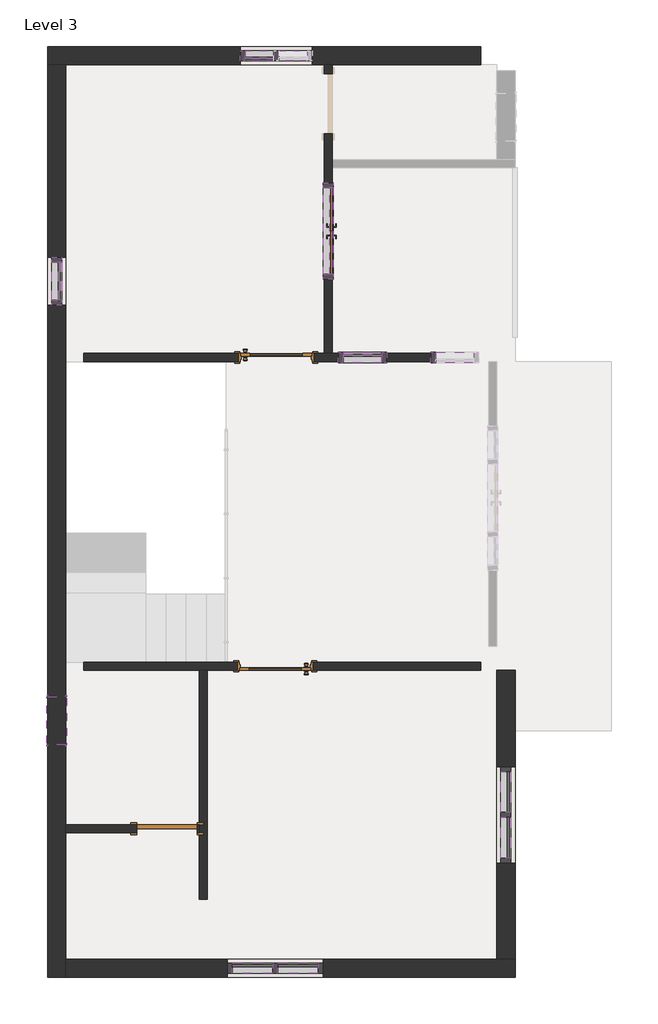
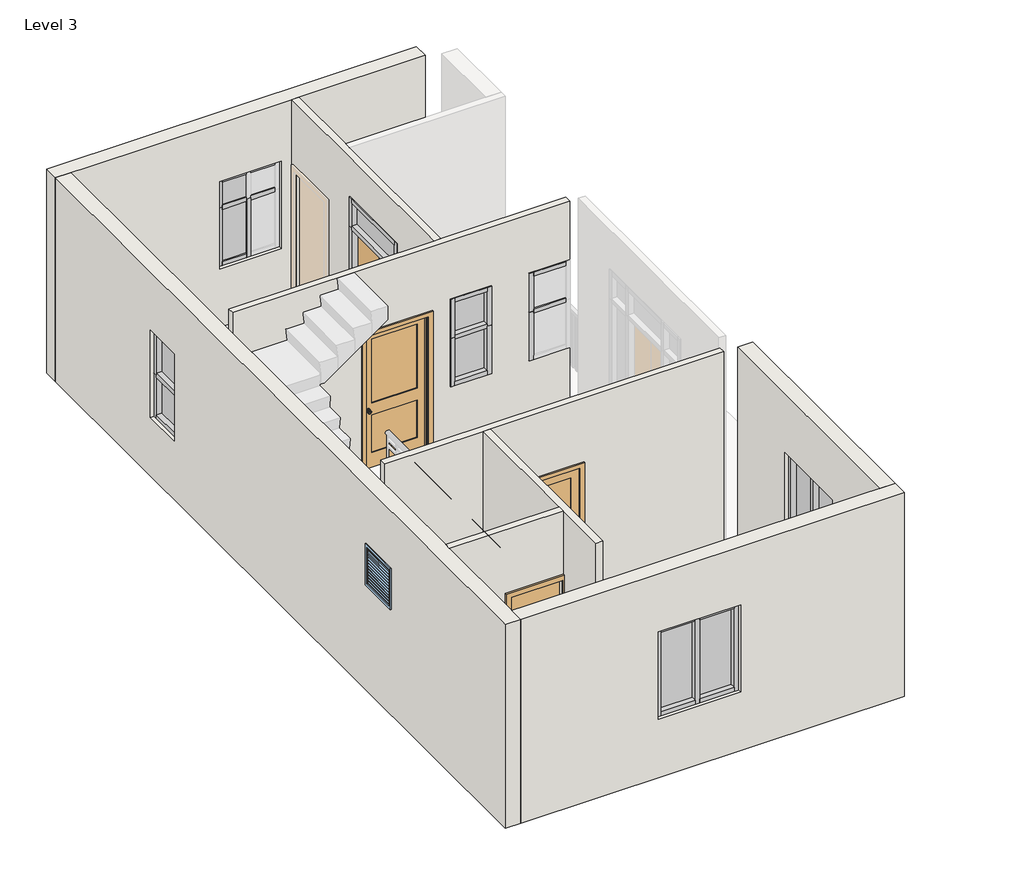
# One storey, part 1 of 2: 47 members, 11 plates, 9 walls, 4 doors, 1 window.
"""IFC4 building model written with IfcOpenShell, lengths in millimetres."""

from ifc_helpers import new_model, si_unit, frame, origin, place, context, project, spatial, polyline, outline, extrude, faceted_brep, transform, mapped, element, save
from components import door_curtain_wall_double_glass_door_curtain_wall_double_295e6296, door_interior_single_2_panel_wood_3_x7_894b38f8, door_270f2424, member_0b7646a3, member_15823cb3, member_843225dc, member_af2f84b9, member_3374d9b6, member_273a15f2, member_867fe1e1, member_86d06fe4, member_323df77c, member_47bfaf8a, member_aa870034, member_824a4a8d, member_c6627131, member_410c6227, member_73c23c35, member_6e28d7e1, system_panel_glazed_235599b7, system_panel_glazed_a38391a9, system_panel_glazed_afbb4b88, system_panel_glazed_c43f0a09, system_panel_glazed_df5e78e0, system_panel_glazed_cc98a0ec, system_panel_glazed_2bcfbbac, window_f2d8fef0

model = new_model("IFC4")

# Units and contexts
model_context = context("Model", 3, world=origin())
ifc_project = project(units=[si_unit("LENGTHUNIT", "METRE", prefix="MILLI")], contexts=[model_context])

# Site, building, storey
site = spatial("IfcSite", under=ifc_project)
building = spatial("IfcBuilding", under=site)
storey = spatial("IfcBuildingStorey", under=building, Name="Level 3", Elevation=3810.0)

# Doors
placement = place(None, origin())
door_curtain_wall_double_glass_door_curtain_wall_double_shape = door_curtain_wall_double_glass_door_curtain_wall_double_295e6296(model_context)
element("IfcDoor", 1, ObjectType="Door-Curtain-Wall-Double-Glass : Door-Curtain-Wall-Double-Glass", at=placement, inside=storey, context=model_context, shape_type="MappedRepresentation", body=[
    mapped(door_curtain_wall_double_glass_door_curtain_wall_double_shape, transform((-1506.3165653, 5261.1857557, 3873.5), x_axis=(0.0, -1.0, 0.0), y_axis=(1.0, 0.0, 0.0), z_axis=(0.0, 0.0, 1.0))),
])
door_interior_single_2_panel_wood_3_x7_shape = door_interior_single_2_panel_wood_3_x7_894b38f8(model_context)
element("IfcDoor", 2, ObjectType="Door-Interior-Single-2_Panel-Wood : 3'x7'", at=placement, inside=storey, context=model_context, shape_type="MappedRepresentation", body=[
    mapped(door_interior_single_2_panel_wood_3_x7_shape, transform((-2166.7165653, 3664.1607557, 3810.0), x_axis=(1.0, 0.0, 0.0), y_axis=(0.0, 1.0, 0.0), z_axis=(0.0, 0.0, 1.0))),
])
element("IfcDoor", 3, ObjectType="Door-Interior-Single-2_Panel-Wood : 3'x7'", at=placement, inside=storey, context=model_context, shape_type="MappedRepresentation", body=[
    mapped(door_interior_single_2_panel_wood_3_x7_shape, transform((-2179.4165653, -253.7892443, 3810.0), x_axis=(-1.0, 0.0, 0.0), y_axis=(0.0, -1.0, 0.0), z_axis=(0.0, 0.0, 1.0))),
])
door_shape = door_270f2424(model_context)
element("IfcDoor", 4, ObjectType="Single-Flush : 2'6\" x7'", at=placement, inside=storey, context=model_context, shape_type="MappedRepresentation", body=[
    mapped(door_shape, transform((-3551.0165653, -2308.0142443, 3810.0), x_axis=(1.0, 0.0, 0.0), y_axis=(0.0, 1.0, 0.0), z_axis=(0.0, 0.0, 1.0))),
])

# Members
member_shape = member_0b7646a3(model_context)
element("IfcMember", 5, ObjectType="Rectangular Mullion : 2.5\" x 5\" rectangular", at=placement, inside=storey, context=model_context, shape_type="MappedRepresentation", body=[
    mapped(member_shape, transform((741.5834347, -2676.3142441, 6096.0), x_axis=(0.0, 0.0, 1.0), y_axis=(-1.0, 0.0, 0.0), z_axis=(0.0, -1.0, 0.0))),
])
element("IfcMember", 6, ObjectType="Rectangular Mullion : 2.5\" x 5\" rectangular", at=placement, inside=storey, context=model_context, shape_type="MappedRepresentation", body=[
    mapped(member_shape, transform((741.5834347, -2098.4642441, 6096.0), x_axis=(0.0, 0.0, 1.0), y_axis=(-1.0, 0.0, 0.0), z_axis=(0.0, -1.0, 0.0))),
])
element("IfcMember", 7, ObjectType="Rectangular Mullion : 2.5\" x 5\" rectangular", at=placement, inside=storey, context=model_context, shape_type="MappedRepresentation", body=[
    mapped(member_shape, transform((-1633.3165653, -4073.3142443, 6096.0), x_axis=(0.0, 0.0, 1.0), y_axis=(0.0, -1.0, 0.0), z_axis=(1.0, 0.0, 0.0))),
])
element("IfcMember", 8, ObjectType="Rectangular Mullion : 2.5\" x 5\" rectangular", at=placement, inside=storey, context=model_context, shape_type="MappedRepresentation", body=[
    mapped(member_shape, transform((-2211.1665653, -4073.3142443, 6096.0), x_axis=(0.0, 0.0, 1.0), y_axis=(0.0, -1.0, 0.0), z_axis=(1.0, 0.0, 0.0))),
])
element("IfcMember", 9, ObjectType="Rectangular Mullion : 2.5\" x 5\" rectangular", at=placement, inside=storey, context=model_context, shape_type="MappedRepresentation", body=[
    mapped(member_shape, transform((741.5834347, -1584.1142441, 4724.4), x_axis=(0.0, 0.0, -1.0), y_axis=(-1.0, 0.0, 0.0), z_axis=(0.0, 1.0, 0.0))),
])
element("IfcMember", 10, ObjectType="Rectangular Mullion : 2.5\" x 5\" rectangular", at=placement, inside=storey, context=model_context, shape_type="MappedRepresentation", body=[
    mapped(member_shape, transform((741.5834347, -2161.9642441, 4724.4), x_axis=(0.0, 0.0, -1.0), y_axis=(-1.0, 0.0, 0.0), z_axis=(0.0, 1.0, 0.0))),
])
element("IfcMember", 11, ObjectType="Rectangular Mullion : 2.5\" x 5\" rectangular", at=placement, inside=storey, context=model_context, shape_type="MappedRepresentation", body=[
    mapped(member_shape, transform((-2725.5165653, -4073.3142443, 4724.4), x_axis=(0.0, 0.0, -1.0), y_axis=(0.0, -1.0, 0.0), z_axis=(-1.0, 0.0, 0.0))),
])
element("IfcMember", 12, ObjectType="Rectangular Mullion : 2.5\" x 5\" rectangular", at=placement, inside=storey, context=model_context, shape_type="MappedRepresentation", body=[
    mapped(member_shape, transform((-2147.6665653, -4073.3142443, 4724.4), x_axis=(0.0, 0.0, -1.0), y_axis=(0.0, -1.0, 0.0), z_axis=(-1.0, 0.0, 0.0))),
])
member_2_shape = member_15823cb3(model_context)
element("IfcMember", 13, ObjectType="Rectangular Mullion : 2.5\" x 5\" rectangular", at=placement, inside=storey, context=model_context, shape_type="MappedRepresentation", body=[
    mapped(member_2_shape, transform((-1506.3165653, 5870.7857557, 6400.8), x_axis=(0.0, 1.0, 0.0), y_axis=(-1.0, 0.0, 0.0), z_axis=(0.0, 0.0, 1.0))),
])
element("IfcMember", 14, ObjectType="Rectangular Mullion : 2.5\" x 5\" rectangular", at=placement, inside=storey, context=model_context, shape_type="MappedRepresentation", body=[
    mapped(member_2_shape, transform((-1506.3165653, 4651.5857557, 5943.6), x_axis=(0.0, -1.0, 0.0), y_axis=(-1.0, 0.0, 0.0), z_axis=(0.0, 0.0, -1.0))),
])
element("IfcMember", 15, ObjectType="Rectangular Mullion : 2.5\" x 5\" rectangular", at=placement, inside=storey, context=model_context, shape_type="MappedRepresentation", body=[
    mapped(member_2_shape, transform((-2623.9165653, 7483.6857557, 5638.8), x_axis=(-1.0, 0.0, 0.0), y_axis=(0.0, 1.0, 0.0), z_axis=(0.0, 0.0, -1.0))),
])
member_3_shape = member_843225dc(model_context)
element("IfcMember", 16, ObjectType="Rectangular Mullion : 2.5\" x 5\" rectangular", at=placement, inside=storey, context=model_context, shape_type="MappedRepresentation", body=[
    mapped(member_3_shape, transform((-2560.4165653, 7483.6857557, 6096.0), x_axis=(0.0, 0.0, 1.0), y_axis=(0.0, 1.0, 0.0), z_axis=(-1.0, 0.0, 0.0))),
])
element("IfcMember", 17, ObjectType="Rectangular Mullion : 2.5\" x 5\" rectangular", at=placement, inside=storey, context=model_context, shape_type="MappedRepresentation", body=[
    mapped(member_3_shape, transform((-2134.9665653, 7483.6857557, 6096.0), x_axis=(0.0, 0.0, 1.0), y_axis=(0.0, 1.0, 0.0), z_axis=(-1.0, 0.0, 0.0))),
])
element("IfcMember", 18, ObjectType="Rectangular Mullion : 2.5\" x 5\" rectangular", at=placement, inside=storey, context=model_context, shape_type="MappedRepresentation", body=[
    mapped(member_3_shape, transform((-2198.4665653, 7483.6857557, 4724.4), x_axis=(0.0, 0.0, -1.0), y_axis=(0.0, 1.0, 0.0), z_axis=(1.0, 0.0, 0.0))),
])
member_4_shape = member_af2f84b9(model_context)
element("IfcMember", 19, ObjectType="Rectangular Mullion : 2.5\" x 5\" rectangular", at=placement, inside=storey, context=model_context, shape_type="MappedRepresentation", body=[
    mapped(member_4_shape, transform((-2134.9665653, 7483.6857557, 5638.8), x_axis=(0.0, 0.0, 1.0), y_axis=(0.0, 1.0, 0.0), z_axis=(-1.0, 0.0, 0.0))),
])
element("IfcMember", 20, ObjectType="Rectangular Mullion : 2.5\" x 5\" rectangular", at=placement, inside=storey, context=model_context, shape_type="MappedRepresentation", body=[
    mapped(member_4_shape, transform((-2560.4165653, 7483.6857557, 5638.8), x_axis=(0.0, 0.0, 1.0), y_axis=(0.0, 1.0, 0.0), z_axis=(-1.0, 0.0, 0.0))),
])
member_5_shape = member_3374d9b6(model_context)
element("IfcMember", 21, ObjectType="Rectangular Mullion : 2.5\" x 5\" rectangular", at=placement, inside=storey, context=model_context, shape_type="MappedRepresentation", body=[
    mapped(member_5_shape, transform((-1506.3165653, 4651.5857557, 3810.0), x_axis=(0.0, -1.0, 0.0), y_axis=(-1.0, 0.0, 0.0), z_axis=(0.0, 0.0, -1.0))),
])
element("IfcMember", 22, ObjectType="Rectangular Mullion : 2.5\" x 5\" rectangular", at=placement, inside=storey, context=model_context, shape_type="MappedRepresentation", body=[
    mapped(member_5_shape, transform((-1506.3165653, 5870.7857557, 5943.6), x_axis=(0.0, 1.0, 0.0), y_axis=(-1.0, 0.0, 0.0), z_axis=(0.0, 0.0, 1.0))),
])
member_6_shape = member_273a15f2(model_context)
element("IfcMember", 23, ObjectType="Rectangular Mullion : 2.5\" x 5\" rectangular", at=placement, inside=storey, context=model_context, shape_type="MappedRepresentation", body=[
    mapped(member_6_shape, transform((-1506.3165653, 4715.0857557, 6400.8), x_axis=(0.0, 0.0, 1.0), y_axis=(-1.0, 0.0, 0.0), z_axis=(0.0, -1.0, 0.0))),
])
element("IfcMember", 24, ObjectType="Rectangular Mullion : 2.5\" x 5\" rectangular", at=placement, inside=storey, context=model_context, shape_type="MappedRepresentation", body=[
    mapped(member_6_shape, transform((-1506.3165653, 5807.2857557, 3810.0), x_axis=(0.0, 0.0, -1.0), y_axis=(-1.0, 0.0, 0.0), z_axis=(0.0, 1.0, 0.0))),
])
member_7_shape = member_867fe1e1(model_context)
element("IfcMember", 25, ObjectType="Rectangular Mullion : 2.5\" x 5\" rectangular", at=placement, inside=storey, context=model_context, shape_type="MappedRepresentation", body=[
    mapped(member_7_shape, transform((-1506.3165653, 4715.0857557, 5943.6), x_axis=(0.0, 0.0, 1.0), y_axis=(-1.0, 0.0, 0.0), z_axis=(0.0, -1.0, 0.0))),
])
member_8_shape = member_86d06fe4(model_context)
element("IfcMember", 26, ObjectType="Rectangular Mullion : 2.5\" x 5\" rectangular", at=placement, inside=storey, context=model_context, shape_type="MappedRepresentation", body=[
    mapped(member_8_shape, transform((-147.4165653, 3660.9857557, 6096.0), x_axis=(0.0, 0.0, 1.0), y_axis=(0.0, 1.0, 0.0), z_axis=(-1.0, 0.0, 0.0))),
])
element("IfcMember", 27, ObjectType="Rectangular Mullion : 2.5\" x 5\" rectangular", at=placement, inside=storey, context=model_context, shape_type="MappedRepresentation", body=[
    mapped(member_8_shape, transform((-833.2165653, 3660.9857557, 6096.0), x_axis=(0.0, 0.0, 1.0), y_axis=(0.0, -1.0, 0.0), z_axis=(1.0, 0.0, 0.0))),
])
element("IfcMember", 28, ObjectType="Rectangular Mullion : 2.5\" x 5\" rectangular", at=placement, inside=storey, context=model_context, shape_type="MappedRepresentation", body=[
    mapped(member_8_shape, transform((-4948.0165653, 4384.8857559, 6096.0), x_axis=(0.0, 0.0, 1.0), y_axis=(-1.0, 0.0, 0.0), z_axis=(0.0, -1.0, 0.0))),
])
element("IfcMember", 29, ObjectType="Rectangular Mullion : 2.5\" x 5\" rectangular", at=placement, inside=storey, context=model_context, shape_type="MappedRepresentation", body=[
    mapped(member_8_shape, transform((-1315.8165653, 3660.9857557, 4724.4), x_axis=(0.0, 0.0, -1.0), y_axis=(0.0, -1.0, 0.0), z_axis=(-1.0, 0.0, 0.0))),
])
element("IfcMember", 30, ObjectType="Rectangular Mullion : 2.5\" x 5\" rectangular", at=placement, inside=storey, context=model_context, shape_type="MappedRepresentation", body=[
    mapped(member_8_shape, transform((-4948.0165653, 4867.4857559, 4724.4), x_axis=(0.0, 0.0, -1.0), y_axis=(-1.0, 0.0, 0.0), z_axis=(0.0, 1.0, 0.0))),
])
member_9_shape = member_323df77c(model_context)
element("IfcMember", 31, ObjectType="Rectangular Mullion : 2.5\" x 5\" rectangular", at=placement, inside=storey, context=model_context, shape_type="MappedRepresentation", body=[
    mapped(member_9_shape, transform((-147.4165653, 3660.9857557, 5486.4), x_axis=(0.0, 0.0, 1.0), y_axis=(0.0, 1.0, 0.0), z_axis=(-1.0, 0.0, 0.0))),
])
element("IfcMember", 32, ObjectType="Rectangular Mullion : 2.5\" x 5\" rectangular", at=placement, inside=storey, context=model_context, shape_type="MappedRepresentation", body=[
    mapped(member_9_shape, transform((-833.2165653, 3660.9857557, 5486.4), x_axis=(0.0, 0.0, 1.0), y_axis=(0.0, -1.0, 0.0), z_axis=(1.0, 0.0, 0.0))),
])
element("IfcMember", 33, ObjectType="Rectangular Mullion : 2.5\" x 5\" rectangular", at=placement, inside=storey, context=model_context, shape_type="MappedRepresentation", body=[
    mapped(member_9_shape, transform((-4948.0165653, 4384.8857559, 5410.2), x_axis=(0.0, 0.0, 1.0), y_axis=(-1.0, 0.0, 0.0), z_axis=(0.0, -1.0, 0.0))),
])
member_10_shape = member_47bfaf8a(model_context)
element("IfcMember", 34, ObjectType="Rectangular Mullion : 2.5\" x 5\" rectangular", at=placement, inside=storey, context=model_context, shape_type="MappedRepresentation", body=[
    mapped(member_10_shape, transform((-1379.3165653, 3660.9857557, 6096.0), x_axis=(-1.0, 0.0, 0.0), y_axis=(0.0, -1.0, 0.0), z_axis=(0.0, 0.0, 1.0))),
])
member_11_shape = member_aa870034(model_context)
element("IfcMember", 35, ObjectType="Rectangular Mullion : 2.5\" x 5\" rectangular", at=placement, inside=storey, context=model_context, shape_type="MappedRepresentation", body=[
    mapped(member_11_shape, transform((-210.9165653, 3660.9857557, 4724.4), x_axis=(-1.0, 0.0, 0.0), y_axis=(0.0, 1.0, 0.0), z_axis=(0.0, 0.0, -1.0))),
])
element("IfcMember", 36, ObjectType="Rectangular Mullion : 2.5\" x 5\" rectangular", at=placement, inside=storey, context=model_context, shape_type="MappedRepresentation", body=[
    mapped(member_11_shape, transform((-769.7165653, 3660.9857557, 4724.4), x_axis=(1.0, 0.0, 0.0), y_axis=(0.0, -1.0, 0.0), z_axis=(0.0, 0.0, -1.0))),
])
element("IfcMember", 37, ObjectType="Rectangular Mullion : 2.5\" x 5\" rectangular", at=placement, inside=storey, context=model_context, shape_type="MappedRepresentation", body=[
    mapped(member_10_shape, transform((-210.9165653, 3660.9857557, 5486.4), x_axis=(-1.0, 0.0, 0.0), y_axis=(0.0, 1.0, 0.0), z_axis=(0.0, 0.0, -1.0))),
])
element("IfcMember", 38, ObjectType="Rectangular Mullion : 2.5\" x 5\" rectangular", at=placement, inside=storey, context=model_context, shape_type="MappedRepresentation", body=[
    mapped(member_10_shape, transform((-769.7165653, 3660.9857557, 5486.4), x_axis=(1.0, 0.0, 0.0), y_axis=(0.0, -1.0, 0.0), z_axis=(0.0, 0.0, -1.0))),
])
element("IfcMember", 39, ObjectType="Rectangular Mullion : 2.5\" x 5\" rectangular", at=placement, inside=storey, context=model_context, shape_type="MappedRepresentation", body=[
    mapped(member_11_shape, transform((-1379.3165653, 3660.9857557, 5486.4), x_axis=(-1.0, 0.0, 0.0), y_axis=(0.0, -1.0, 0.0), z_axis=(0.0, 0.0, 1.0))),
])
member_12_shape = member_824a4a8d(model_context)
element("IfcMember", 40, ObjectType="Rectangular Mullion : 2.5\" x 5\" rectangular", at=placement, inside=storey, context=model_context, shape_type="MappedRepresentation", body=[
    mapped(member_12_shape, transform((741.5834347, -2130.2142441, 4724.4), x_axis=(0.0, -1.0, 0.0), y_axis=(-1.0, 0.0, 0.0), z_axis=(0.0, 0.0, -1.0))),
])
element("IfcMember", 41, ObjectType="Rectangular Mullion : 2.5\" x 5\" rectangular", at=placement, inside=storey, context=model_context, shape_type="MappedRepresentation", body=[
    mapped(member_12_shape, transform((-2179.4165653, -4073.3142443, 4724.4), x_axis=(1.0, 0.0, 0.0), y_axis=(0.0, -1.0, 0.0), z_axis=(0.0, 0.0, -1.0))),
])
member_13_shape = member_c6627131(model_context)
element("IfcMember", 42, ObjectType="Rectangular Mullion : 2.5\" x 5\" rectangular", at=placement, inside=storey, context=model_context, shape_type="MappedRepresentation", body=[
    mapped(member_13_shape, transform((741.5834347, -1520.6142441, 6096.0), x_axis=(0.0, 1.0, 0.0), y_axis=(-1.0, 0.0, 0.0), z_axis=(0.0, 0.0, 1.0))),
])
element("IfcMember", 43, ObjectType="Rectangular Mullion : 2.5\" x 5\" rectangular", at=placement, inside=storey, context=model_context, shape_type="MappedRepresentation", body=[
    mapped(member_13_shape, transform((-2789.0165653, -4073.3142443, 6096.0), x_axis=(-1.0, 0.0, 0.0), y_axis=(0.0, -1.0, 0.0), z_axis=(0.0, 0.0, 1.0))),
])
element("IfcMember", 44, ObjectType="Rectangular Mullion : 2.5\" x 5\" rectangular", at=placement, inside=storey, context=model_context, shape_type="MappedRepresentation", body=[
    mapped(member_13_shape, transform((741.5834347, -2739.8142441, 4724.4), x_axis=(0.0, -1.0, 0.0), y_axis=(-1.0, 0.0, 0.0), z_axis=(0.0, 0.0, -1.0))),
])
element("IfcMember", 45, ObjectType="Rectangular Mullion : 2.5\" x 5\" rectangular", at=placement, inside=storey, context=model_context, shape_type="MappedRepresentation", body=[
    mapped(member_13_shape, transform((-1569.8165653, -4073.3142443, 4724.4), x_axis=(1.0, 0.0, 0.0), y_axis=(0.0, -1.0, 0.0), z_axis=(0.0, 0.0, -1.0))),
])
member_14_shape = member_410c6227(model_context)
element("IfcMember", 46, ObjectType="Rectangular Mullion : 2.5\" x 5\" rectangular", at=placement, inside=storey, context=model_context, shape_type="MappedRepresentation", body=[
    mapped(member_14_shape, transform((-2166.7165653, 7483.6857557, 4724.4), x_axis=(-1.0, 0.0, 0.0), y_axis=(0.0, 1.0, 0.0), z_axis=(0.0, 0.0, -1.0))),
])
member_15_shape = member_73c23c35(model_context)
element("IfcMember", 47, ObjectType="Rectangular Mullion : 2.5\" x 5\" rectangular", at=placement, inside=storey, context=model_context, shape_type="MappedRepresentation", body=[
    mapped(member_15_shape, transform((-2623.9165653, 7483.6857557, 4724.4), x_axis=(-1.0, 0.0, 0.0), y_axis=(0.0, 1.0, 0.0), z_axis=(0.0, 0.0, -1.0))),
])
member_16_shape = member_6e28d7e1(model_context)
element("IfcMember", 48, ObjectType="Rectangular Mullion : 2.5\" x 5\" rectangular", at=placement, inside=storey, context=model_context, shape_type="MappedRepresentation", body=[
    mapped(member_16_shape, transform((-4948.0165653, 4930.9857559, 6096.0), x_axis=(0.0, 1.0, 0.0), y_axis=(-1.0, 0.0, 0.0), z_axis=(0.0, 0.0, 1.0))),
])
element("IfcMember", 49, ObjectType="Rectangular Mullion : 2.5\" x 5\" rectangular", at=placement, inside=storey, context=model_context, shape_type="MappedRepresentation", body=[
    mapped(member_16_shape, transform((-4948.0165653, 4321.3857559, 4724.4), x_axis=(0.0, -1.0, 0.0), y_axis=(-1.0, 0.0, 0.0), z_axis=(0.0, 0.0, -1.0))),
])
element("IfcMember", 50, ObjectType="Rectangular Mullion : 2.5\" x 5\" rectangular", at=placement, inside=storey, context=model_context, shape_type="MappedRepresentation", body=[
    mapped(member_16_shape, transform((-4948.0165653, 4321.3857559, 5410.2), x_axis=(0.0, -1.0, 0.0), y_axis=(-1.0, 0.0, 0.0), z_axis=(0.0, 0.0, -1.0))),
])
element("IfcMember", 51, ObjectType="Rectangular Mullion : 2.5\" x 5\" rectangular", at=placement, inside=storey, context=model_context, shape_type="MappedRepresentation", body=[
    mapped(member_16_shape, transform((-4948.0165653, 4930.9857559, 5410.2), x_axis=(0.0, 1.0, 0.0), y_axis=(-1.0, 0.0, 0.0), z_axis=(0.0, 0.0, 1.0))),
])

# Plates
system_panel_glazed_shape = system_panel_glazed_235599b7(model_context)
element("IfcPlate", 52, ObjectType="System Panel : Glazed", at=placement, inside=storey, context=model_context, shape_type="MappedRepresentation", body=[
    mapped(system_panel_glazed_shape, transform((-2379.4415653, 7483.6857557, 5670.55), x_axis=(-1.0, 0.0, 0.0), y_axis=(0.0, -1.0, 0.0), z_axis=(0.0, 0.0, 1.0))),
])
system_panel_glazed_2_shape = system_panel_glazed_a38391a9(model_context)
element("IfcPlate", 53, ObjectType="System Panel : Glazed", at=placement, inside=storey, context=model_context, shape_type="MappedRepresentation", body=[
    mapped(system_panel_glazed_2_shape, transform((-1506.3165653, 5261.1857557, 5975.35), x_axis=(0.0, -1.0, 0.0), y_axis=(1.0, 0.0, 0.0), z_axis=(0.0, 0.0, 1.0))),
])
system_panel_glazed_3_shape = system_panel_glazed_afbb4b88(model_context)
element("IfcPlate", 54, ObjectType="System Panel : Glazed", at=placement, inside=storey, context=model_context, shape_type="MappedRepresentation", body=[
    mapped(system_panel_glazed_3_shape, transform((-1074.5165653, 3660.9857557, 4787.9), x_axis=(1.0, 0.0, 0.0), y_axis=(0.0, 1.0, 0.0), z_axis=(0.0, 0.0, 1.0))),
])
system_panel_glazed_4_shape = system_panel_glazed_c43f0a09(model_context)
element("IfcPlate", 55, ObjectType="System Panel : Glazed", at=placement, inside=storey, context=model_context, shape_type="MappedRepresentation", body=[
    mapped(system_panel_glazed_4_shape, transform((-1074.5165653, 3660.9857557, 5518.15), x_axis=(1.0, 0.0, 0.0), y_axis=(0.0, 1.0, 0.0), z_axis=(0.0, 0.0, 1.0))),
])
system_panel_glazed_5_shape = system_panel_glazed_df5e78e0(model_context)
element("IfcPlate", 56, ObjectType="System Panel : Glazed", at=placement, inside=storey, context=model_context, shape_type="MappedRepresentation", body=[
    mapped(system_panel_glazed_5_shape, transform((741.5834347, -1841.2892441, 4787.9), x_axis=(0.0, -1.0, 0.0), y_axis=(1.0, 0.0, 0.0), z_axis=(0.0, 0.0, 1.0))),
])
element("IfcPlate", 57, ObjectType="System Panel : Glazed", at=placement, inside=storey, context=model_context, shape_type="MappedRepresentation", body=[
    mapped(system_panel_glazed_5_shape, transform((-2468.3415653, -4073.3142443, 4787.9), x_axis=(1.0, 0.0, 0.0), y_axis=(0.0, 1.0, 0.0), z_axis=(0.0, 0.0, 1.0))),
])
element("IfcPlate", 58, ObjectType="System Panel : Glazed", at=placement, inside=storey, context=model_context, shape_type="MappedRepresentation", body=[
    mapped(system_panel_glazed_5_shape, transform((-1890.4915653, -4073.3142443, 4787.9), x_axis=(1.0, 0.0, 0.0), y_axis=(0.0, 1.0, 0.0), z_axis=(0.0, 0.0, 1.0))),
])
element("IfcPlate", 59, ObjectType="System Panel : Glazed", at=placement, inside=storey, context=model_context, shape_type="MappedRepresentation", body=[
    mapped(system_panel_glazed_5_shape, transform((741.5834347, -2419.1392441, 4787.9), x_axis=(0.0, -1.0, 0.0), y_axis=(1.0, 0.0, 0.0), z_axis=(0.0, 0.0, 1.0))),
])
system_panel_glazed_6_shape = system_panel_glazed_cc98a0ec(model_context)
element("IfcPlate", 60, ObjectType="System Panel : Glazed", at=placement, inside=storey, context=model_context, shape_type="MappedRepresentation", body=[
    mapped(system_panel_glazed_6_shape, transform((-2379.4415653, 7483.6857557, 4787.9), x_axis=(-1.0, 0.0, 0.0), y_axis=(0.0, -1.0, 0.0), z_axis=(0.0, 0.0, 1.0))),
])
system_panel_glazed_7_shape = system_panel_glazed_2bcfbbac(model_context)
element("IfcPlate", 61, ObjectType="System Panel : Glazed", at=placement, inside=storey, context=model_context, shape_type="MappedRepresentation", body=[
    mapped(system_panel_glazed_7_shape, transform((-4948.0165653, 4626.1857559, 4787.9), x_axis=(0.0, -1.0, 0.0), y_axis=(1.0, 0.0, 0.0), z_axis=(0.0, 0.0, 1.0))),
])
element("IfcPlate", 62, ObjectType="System Panel : Glazed", at=placement, inside=storey, context=model_context, shape_type="MappedRepresentation", body=[
    mapped(system_panel_glazed_7_shape, transform((-4948.0165653, 4626.1857559, 5441.95), x_axis=(0.0, -1.0, 0.0), y_axis=(1.0, 0.0, 0.0), z_axis=(0.0, 0.0, 1.0))),
])

# Walls
element("IfcWall", 63, at=placement, inside=storey, context=model_context, shape_type="Brep", body=[
    faceted_brep([(398.6834347, 3610.1857557, 7010.4), (-4605.1165653, 3610.1857557, 7010.4), (-4605.1165653, 3610.1857557, 3810.0), (-2649.3165653, 3610.1857557, 3810.0), (-2649.3165653, 3610.1857557, 5969.0), (-1684.1165653, 3610.1857557, 5969.0), (-1684.1165653, 3610.1857557, 3810.0), (398.6834347, 3610.1857557, 3810.0), (398.6834347, 3610.1857557, 4724.4), (-210.9165653, 3610.1857557, 4724.4), (-210.9165653, 3610.1857557, 6096.0), (398.6834347, 3610.1857557, 6096.0), (-1379.3165653, 3610.1857557, 4724.4), (-1379.3165653, 3610.1857557, 6096.0), (-769.7165653, 3610.1857557, 6096.0), (-769.7165653, 3610.1857557, 4724.4), (-4605.1165653, 3711.7857557, 7010.4), (-1557.1165653, 3711.7857557, 7010.4), (-1455.5165653, 3711.7857557, 7010.4), (398.6834347, 3711.7857557, 7010.4), (398.6834347, 3711.7857557, 6096.0), (-210.9165653, 3711.7857557, 6096.0), (-210.9165653, 3711.7857557, 4724.4), (398.6834347, 3711.7857557, 4724.4), (398.6834347, 3711.7857557, 3810.0), (-1455.5165653, 3711.7857557, 3810.0), (-1557.1165653, 3711.7857557, 3810.0), (-1684.1165653, 3711.7857557, 3810.0), (-1684.1165653, 3711.7857557, 5969.0), (-2649.3165653, 3711.7857557, 5969.0), (-2649.3165653, 3711.7857557, 3810.0), (-4605.1165653, 3711.7857557, 3810.0), (-1379.3165653, 3711.7857557, 6096.0), (-1379.3165653, 3711.7857557, 4724.4), (-769.7165653, 3711.7857557, 4724.4), (-769.7165653, 3711.7857557, 6096.0)], [[[0, 1, 2, 3, 4, 5, 6, 7, 8, 9, 10, 11], [12, 13, 14, 15]], [[16, 17, 18, 19, 20, 21, 22, 23, 24, 25, 26, 27, 28, 29, 30, 31], [32, 33, 34, 35]], [[2, 31, 30, 3]], [[24, 7, 6, 27, 26, 25]], [[7, 24, 23, 8]], [[19, 0, 11, 20]], [[1, 0, 19, 18, 17, 16]], [[2, 1, 16, 31]], [[5, 28, 27, 6]], [[28, 5, 4, 29]], [[29, 4, 3, 30]], [[12, 33, 32, 13]], [[13, 32, 35, 14]], [[34, 15, 14, 35]], [[33, 12, 15, 34]], [[10, 21, 20, 11]], [[21, 10, 9, 22]], [[22, 9, 8, 23]]]),
])
element("IfcWall", 64, at=placement, inside=storey, context=model_context, shape_type="Brep", body=[
    faceted_brep([(424.0834347, -301.4142443, 3810.0), (424.0834347, -301.4142443, 7010.4), (-3043.0165653, -301.4142443, 7010.4), (-3144.6165653, -301.4142443, 7010.4), (-4605.1165653, -301.4142443, 7010.4), (-4605.1165653, -301.4142443, 3810.0), (-3144.6165653, -301.4142443, 3810.0), (-3043.0165653, -301.4142443, 3810.0), (-2662.0165653, -301.4142443, 3810.0), (-2662.0165653, -301.4142443, 5969.0), (-1696.8165653, -301.4142443, 5969.0), (-1696.8165653, -301.4142443, 3810.0), (398.6834347, -301.4142443, 3810.0), (424.0834347, -199.8142443, 7010.4), (424.0834347, -199.8142443, 3810.0), (398.6834347, -199.8142443, 3810.0), (-1696.8165653, -199.8142443, 3810.0), (-1696.8165653, -199.8142443, 5969.0), (-2662.0165653, -199.8142443, 5969.0), (-2662.0165653, -199.8142443, 3810.0), (-4605.1165653, -199.8142443, 3810.0), (-4605.1165653, -199.8142443, 7010.4), (398.6834347, -199.8142443, 7010.4)], [[[0, 1, 2, 3, 4, 5, 6, 7, 8, 9, 10, 11, 12]], [[13, 14, 15, 16, 17, 18, 19, 20, 21, 22]], [[5, 20, 19, 8, 7, 6]], [[14, 0, 12, 11, 16, 15]], [[1, 0, 14, 13]], [[4, 3, 2, 1, 13, 22, 21]], [[5, 4, 21, 20]], [[18, 9, 8, 19]], [[9, 18, 17, 10]], [[10, 17, 16, 11]]]),
])
element("IfcWall", 65, at=placement, inside=storey, context=model_context, shape_type="Brep", body=[
    faceted_brep([(-1455.5165653, 7369.3857557, 7010.4), (-1455.5165653, 6162.8857557, 7010.4), (-1455.5165653, 6061.2857557, 7010.4), (-1455.5165653, 3711.7857557, 7010.4), (-1455.5165653, 3711.7857557, 3810.0), (-1455.5165653, 4651.5857557, 3810.0), (-1455.5165653, 4651.5857557, 6400.8), (-1455.5165653, 5870.7857557, 6400.8), (-1455.5165653, 5870.7857557, 3810.0), (-1455.5165653, 6061.2857557, 3810.0), (-1455.5165653, 6162.8857557, 3810.0), (-1455.5165653, 6493.0857557, 3810.0), (-1455.5165653, 6493.0857557, 5943.6), (-1455.5165653, 7255.0857557, 5943.6), (-1455.5165653, 7255.0857557, 3810.0), (-1455.5165653, 7369.3857557, 3810.0), (-1557.1165653, 3711.7857557, 7010.4), (-1557.1165653, 7369.3857557, 7010.4), (-1557.1165653, 7369.3857557, 3810.0), (-1557.1165653, 7255.0857557, 3810.0), (-1557.1165653, 7255.0857557, 5943.6), (-1557.1165653, 6493.0857557, 5943.6), (-1557.1165653, 6493.0857557, 3810.0), (-1557.1165653, 5870.7857557, 3810.0), (-1557.1165653, 5870.7857557, 6400.8), (-1557.1165653, 4651.5857557, 6400.8), (-1557.1165653, 4651.5857557, 3810.0), (-1557.1165653, 3711.7857557, 3810.0)], [[[0, 1, 2, 3, 4, 5, 6, 7, 8, 9, 10, 11, 12, 13, 14, 15]], [[16, 17, 18, 19, 20, 21, 22, 23, 24, 25, 26, 27]], [[4, 27, 26, 5]], [[18, 15, 14, 19]], [[22, 11, 10, 9, 8, 23]], [[3, 2, 1, 0, 17, 16]], [[4, 3, 16, 27]], [[0, 15, 18, 17]], [[20, 19, 14, 13]], [[21, 20, 13, 12]], [[22, 21, 12, 11]], [[7, 24, 23, 8]], [[24, 7, 6, 25]], [[25, 6, 5, 26]]]),
])
element("IfcWall", 66, at=placement, inside=storey, context=model_context, shape_type="Brep", body=[
    faceted_brep([(-3144.6165653, -301.4142443, 3810.0), (-3144.6165653, -2257.2142443, 3810.0), (-3144.6165653, -2358.8142443, 3810.0), (-3144.6165653, -3197.0142443, 3810.0), (-3144.6165653, -3197.0142443, 7010.4), (-3144.6165653, -2358.8142443, 7010.4), (-3144.6165653, -2257.2142443, 7010.4), (-3144.6165653, -301.4142443, 7010.4), (-3043.0165653, -301.4142443, 3810.0), (-3043.0165653, -301.4142443, 7010.4), (-3043.0165653, -3197.0142443, 7010.4), (-3043.0165653, -3197.0142443, 3810.0)], [[[0, 1, 2, 3, 4, 5, 6, 7]], [[8, 9, 10, 11]], [[3, 2, 1, 0, 8, 11]], [[4, 3, 11, 10]], [[7, 6, 5, 4, 10, 9]], [[0, 7, 9, 8]]]),
])
element("IfcWall", 67, at=placement, inside=storey, context=model_context, shape_type="SweptSolid", body=[
    extrude(outline(polyline([(5943.6, -3170.0165653), (3810.0, -3170.0165653), (3810.0, -3144.6165653), (7010.4, -3144.6165653), (7010.4, -4833.7165653), (3810.0, -4833.7165653), (3810.0, -3932.0165653), (5943.6, -3932.0165653), (5943.6, -3170.0165653)])), frame((0.0, -2358.8142443, 0.0), z_axis=(0.0, 1.0, 0.0), x_axis=(0.0, 0.0, 1.0)), (0.0, 0.0, 1.0), 101.6),
])
element("IfcWall", 68, ObjectType="9\" wall", at=placement, inside=storey, context=model_context, shape_type="Brep", body=[
    faceted_brep([(-5062.3165653, 7369.3857557, 3810.0), (-4833.7165653, 7369.3857557, 3810.0), (-1557.1165653, 7369.3857557, 3810.0), (-1455.5165653, 7369.3857557, 3810.0), (398.6834347, 7369.3857557, 3810.0), (424.0834347, 7369.3857557, 3810.0), (424.0834347, 7369.3857557, 7010.4), (398.6834347, 7369.3857557, 7010.4), (-1455.5165653, 7369.3857557, 7010.4), (-1557.1165653, 7369.3857557, 7010.4), (-4605.1165653, 7369.3857557, 7010.4), (-4833.7165653, 7369.3857557, 7010.4), (-5062.3165653, 7369.3857557, 7010.4), (-1709.5165653, 7369.3857557, 6096.0), (-1709.5165653, 7369.3857557, 4724.4), (-2623.9165653, 7369.3857557, 4724.4), (-2623.9165653, 7369.3857557, 6096.0), (424.0834347, 7597.9857557, 3810.0), (398.6834347, 7597.9857557, 3810.0), (-5062.3165653, 7597.9857557, 3810.0), (-5062.3165653, 7597.9857557, 7010.4), (424.0834347, 7597.9857557, 7010.4), (-1709.5165653, 7597.9857557, 4724.4), (-1709.5165653, 7597.9857557, 6096.0), (-2623.9165653, 7597.9857557, 6096.0), (-2623.9165653, 7597.9857557, 4724.4)], [[[0, 1, 2, 3, 4, 5, 6, 7, 8, 9, 10, 11, 12], [13, 14, 15, 16]], [[17, 18, 19, 20, 21], [22, 23, 24, 25]], [[5, 4, 3, 2, 1, 0, 19, 18, 17]], [[6, 5, 17, 21]], [[12, 11, 10, 9, 8, 7, 6, 21, 20]], [[0, 12, 20, 19]], [[22, 14, 13, 23]], [[23, 13, 16, 24]], [[24, 16, 15, 25]], [[14, 22, 25, 15]]]),
])
element("IfcWall", 69, ObjectType="9\" wall", at=placement, inside=storey, context=model_context, shape_type="Brep", body=[
    faceted_brep([(-5062.3165653, 7369.3857557, 3810.0), (-5062.3165653, -4187.6142443, 3810.0), (-5062.3165653, -4187.6142443, 7010.4), (-5062.3165653, 7369.3857557, 7010.4), (-5062.3165653, 4930.9857559, 4724.4), (-5062.3165653, 4930.9857559, 6096.0), (-5062.3165653, 4321.3857559, 6096.0), (-5062.3165653, 4321.3857559, 4724.4), (-5062.3165653, -1241.2142443, 6096.0), (-5062.3165653, -1241.2142443, 5486.4), (-5062.3165653, -631.6142443, 5486.4), (-5062.3165653, -631.6142443, 6096.0), (-4833.7165653, -4187.6142443, 3810.0), (-4833.7165653, -3959.0142443, 3810.0), (-4833.7165653, -2358.8142443, 3810.0), (-4833.7165653, -2257.2142443, 3810.0), (-4833.7165653, -301.4142443, 3810.0), (-4833.7165653, -199.8142443, 3810.0), (-4833.7165653, 3610.1857557, 3810.0), (-4833.7165653, 3711.7857557, 3810.0), (-4833.7165653, 7369.3857557, 3810.0), (-4833.7165653, 7369.3857557, 7010.4), (-4833.7165653, 7293.1857557, 7010.4), (-4833.7165653, 3914.9857557, 7010.4), (-4833.7165653, 3610.1857557, 7010.4), (-4833.7165653, 3.3857557, 7010.4), (-4833.7165653, -301.4142443, 7010.4), (-4833.7165653, -2257.2142443, 7010.4), (-4833.7165653, -2358.8142443, 7010.4), (-4833.7165653, -3882.8142443, 7010.4), (-4833.7165653, -3959.0142443, 7010.4), (-4833.7165653, -4187.6142443, 7010.4), (-4833.7165653, 4930.9857559, 6096.0), (-4833.7165653, 4930.9857559, 4724.4), (-4833.7165653, 4321.3857559, 4724.4), (-4833.7165653, 4321.3857559, 6096.0), (-4833.7165653, -1241.2142443, 6096.0), (-4833.7165653, -631.6142443, 6096.0), (-4833.7165653, -631.6142443, 5486.4), (-4833.7165653, -1241.2142443, 5486.4)], [[[0, 1, 2, 3], [4, 5, 6, 7], [8, 9, 10, 11]], [[12, 13, 14, 15, 16, 17, 18, 19, 20, 21, 22, 23, 24, 25, 26, 27, 28, 29, 30, 31], [32, 33, 34, 35], [36, 37, 38, 39]], [[1, 0, 20, 19, 18, 17, 16, 15, 14, 13, 12]], [[3, 2, 31, 30, 29, 28, 27, 26, 25, 24, 23, 22, 21]], [[2, 1, 12, 31]], [[0, 3, 21, 20]], [[4, 33, 32, 5]], [[5, 32, 35, 6]], [[6, 35, 34, 7]], [[33, 4, 7, 34]], [[9, 8, 36, 39]], [[10, 9, 39, 38]], [[11, 10, 38, 37]], [[8, 11, 37, 36]]]),
])
element("IfcWall", 70, ObjectType="9\" wall", at=placement, inside=storey, context=model_context, shape_type="Brep", body=[
    faceted_brep([(-4833.7165653, -4187.6142443, 3810.0), (855.8834347, -4187.6142443, 3810.0), (855.8834347, -4187.6142443, 7010.4), (-4833.7165653, -4187.6142443, 7010.4), (-2789.0165653, -4187.6142443, 4724.4), (-2789.0165653, -4187.6142443, 6096.0), (-1569.8165653, -4187.6142443, 6096.0), (-1569.8165653, -4187.6142443, 4724.4), (855.8834347, -3959.0142443, 3810.0), (627.2834347, -3959.0142443, 3810.0), (-4833.7165653, -3959.0142443, 3810.0), (-4833.7165653, -3959.0142443, 7010.4), (-4605.1165653, -3959.0142443, 7010.4), (398.6834347, -3959.0142443, 7010.4), (627.2834347, -3959.0142443, 7010.4), (855.8834347, -3959.0142443, 7010.4), (-2789.0165653, -3959.0142443, 6096.0), (-2789.0165653, -3959.0142443, 4724.4), (-1569.8165653, -3959.0142443, 4724.4), (-1569.8165653, -3959.0142443, 6096.0)], [[[0, 1, 2, 3], [4, 5, 6, 7]], [[8, 9, 10, 11, 12, 13, 14, 15], [16, 17, 18, 19]], [[1, 0, 10, 9, 8]], [[3, 2, 15, 14, 13, 12, 11]], [[0, 3, 11, 10]], [[2, 1, 8, 15]], [[4, 17, 16, 5]], [[5, 16, 19, 6]], [[6, 19, 18, 7]], [[17, 4, 7, 18]]]),
])
element("IfcWall", 71, ObjectType="9\" wall", at=placement, inside=storey, context=model_context, shape_type="Brep", body=[
    faceted_brep([(855.8834347, -3959.0142443, 3810.0), (855.8834347, -3882.8142443, 3810.0), (855.8834347, -301.4142443, 3810.0), (855.8834347, -301.4142443, 7010.4), (855.8834347, -3959.0142443, 7010.4), (855.8834347, -1520.6142441, 6096.0), (855.8834347, -1520.6142441, 4724.4), (855.8834347, -2739.8142441, 4724.4), (855.8834347, -2739.8142441, 6096.0), (627.2834347, -301.4142443, 3810.0), (627.2834347, -3882.8142443, 3810.0), (627.2834347, -3959.0142443, 3810.0), (627.2834347, -3959.0142443, 7010.4), (627.2834347, -3882.8142443, 7010.4), (627.2834347, -301.4142443, 7010.4), (627.2834347, -1520.6142441, 4724.4), (627.2834347, -1520.6142441, 6096.0), (627.2834347, -2739.8142441, 6096.0), (627.2834347, -2739.8142441, 4724.4)], [[[0, 1, 2, 3, 4], [5, 6, 7, 8]], [[9, 10, 11, 12, 13, 14], [15, 16, 17, 18]], [[2, 1, 0, 11, 10, 9]], [[3, 2, 9, 14]], [[4, 3, 14, 13, 12]], [[0, 4, 12, 11]], [[15, 6, 5, 16]], [[16, 5, 8, 17]], [[17, 8, 7, 18]], [[6, 15, 18, 7]]]),
])

# Window
window_shape = window_f2d8fef0(model_context)
element("IfcWindow", 72, ObjectType="Window-Louvers : 24\" x 24\"", at=placement, inside=storey, context=model_context, shape_type="MappedRepresentation", body=[
    mapped(window_shape, transform((-4954.3665653, -936.4142443, 4572.0), x_axis=(0.0, 1.0, 0.0), y_axis=(-1.0, 0.0, 0.0), z_axis=(0.0, 0.0, 1.0))),
])

save(model, "model.ifc")

# Revit data of these elements
# Type "Door-Curtain-Wall-Double-Glass : Door-Curtain-Wall-Double-Glass"
#   Type Mark = "16"
#   Assembly Code = "B2030100"
#   Analytic Construction = "<None>"
#   Width [instance default] = 6' - 0"
#   Thermal Resistance (R) = 10.0000 (h·ft²·°F)/BTU
#   Swing Angle [instance default] = 90.00°
#   Panel Width [instance default] = 3' - 0"
#   Offset = 0' - 2"
#   Heat Transfer Coefficient (U) = 0.1000 BTU/(h·ft²·°F)
#   Define Thermal Properties by = 1
#   Function = 1
#   Door Handle Material = Aluminum
#   Glazing = Glass
#   Visual Light Transmittance = 0
#   Solar Heat Gain Coefficient = 0
#   Construction Type Id = ""
# Type "Door-Interior-Single-2_Panel-Wood : 3'x7'"
#   Type Mark = "9"
#   Assembly Code = "C1020300"
#   Analytic Construction = "Wooden"
#   Top Rail = 0' - 4 11/16"
#   Thickness = 0' - 1 3/8"
#   Thermal Resistance (R) = 2.5876 (h·ft²·°F)/BTU
#   Swing Angle [instance default] = 90.00°
#   Stiles = 0' - 4 3/4"
#   Rough Width = 3' - 2"
#   Rough Height = 7' - 1"
#   Lock Rail = 0' - 7 1/2"
#   Height = 7' - 0"
#   Width = 3' - 0"
#   Heat Transfer Coefficient (U) = 0.3865 BTU/(h·ft²·°F)
#   Bottom Rail = 0' - 9 1/8"
#   Trim Material = Cherry
#   Panel Material = Cherry
#   Frame Material = Cherry
#   Door Handle Material = Aluminum
#   Visual Light Transmittance = 0
#   Solar Heat Gain Coefficient = 0
#   Wall Closure = (empty or 0)
#   Function = (empty or 0)
# Type "Single-Flush : 2'6\" x7'"
#   Type Mark = "15"
#   Construction Type Id = "MDOOR"
#   Assembly Code = "C1020"
#   Analytic Construction = "Metal"
#   Thickness = 0' - 2"
#   Heat Transfer Coefficient (U) = 0.651978 BTU/(h·ft²·°F)
#   Height = 7' - 0"
#   Trim Projection Ext = 0' - 1"
#   Trim Projection Int = 0' - 1"
#   Trim Width = 0' - 3"
#   Width = 2' - 6"
#   Define Thermal Properties by = 1
#   Door Material = Door - Panel
#   Frame Material = Door - Frame
#   Visual Light Transmittance = 0
#   Solar Heat Gain Coefficient = 0
#   Function = (empty or 0)
#   Wall Closure = (empty or 0)
# Type "Rectangular Mullion : 2.5\" x 5\" rectangular"
#   built-in parameter 1007304 = 0.416667 (stored number, unit not read)
#   built-in parameter 1007301 = 0.104167 (stored number, unit not read)
#   built-in parameter 1007300 = 0.104167 (stored number, unit not read)
# Type "System Panel : Glazed"
#   Construction Type Id = "GSP4R"
#   Analytic Construction = "1/8 in Pilkington single glazing"
#   Visual Light Transmittance = 0.9
#   Solar Heat Gain Coefficient = 0.86
#   Heat Transfer Coefficient (U) = 1.18115 BTU/(h·ft²·°F)
#   Define Thermal Properties by = 1
# Type
#   Assembly Code = "B2010"
#   Layers, outside or top first: 0' - 4" "01-9\" wall" (function 1)
# Type "9\" wall"
#   Assembly Code = "B2010"
#   Layers, outside or top first: 0' - 9" "01-9\" wall" (function 1)
# Type "Window-Louvers : 24\" x 24\""
#   Type Mark = "18"
#   Construction Type Id = "GSP4R"
#   Assembly Code = "B20"
#   Analytic Construction = "1/8 in Pilkington single glazing"
#   Visual Light Transmittance = 0.9
#   Thermal Resistance (R) = 1.53941 (h·ft²·°F)/BTU
#   Solar Heat Gain Coefficient = 0.78
#   Max Height = 1' - 11.74264"
#   Height = 2' - 0"
#   Heat Transfer Coefficient (U) = 0.6496 BTU/(h·ft²·°F)
#   Blade Width [instance default] = 1' - 10 1/2"
#   Blade Vertical Thickness = 0' - 0.35355"
#   Blade Thickness = 0' - 0 1/4"
#   Blade Spacing = 0' - 1 1/2"
#   Blade Height = 0' - 1.85355"
#   Blade Depth = 0' - 3"
#   Blade Angle = 45.00°
#   Default Sill Height = 3' - 0"
#   Trim Projection_Exterior = 0' - 0 1/2"
#   Trim Projection_Interior = 0' - 0 1/2"
#   Trim Width_Exterior = 0' - 1 1/2"
#   Trim Width_Interior = 0' - 1 1/2"
#   Width = 2' - 0"
#   Max Blade Count = 12
#   Define Thermal Properties by = 1
#   Blade Count = 12
#   Frame Material = Birch
#   Louver Material = Birch
#   Trim Exterior Material = Birch
#   Trim Interior Material = Birch
#   Wall Closure = (empty or 0)
# Element 1 (IfcDoor, "Door-Curtain-Wall-Double-Glass : Door-Curtain-Wall-Double-Glass")
#   Swing Angle = 90.00°
#   Phase Created = New Construction
#   Materials on its faces: "Aluminum", "Glass"
# Elements 2, 3 (IfcDoor, "Door-Interior-Single-2_Panel-Wood : 3'x7'")
#   Swing Angle = 90.00°
#   Phase Created = New Construction
#   Materials on its faces: "Cherry", "Aluminum"
# Element 4 (IfcDoor, "Single-Flush : 2'6\" x7'")
#   Phase Created = New Construction
#   Materials on its faces: "Door - Frame", "Door - Panel"
# Elements 5, 6, 7, 8, 9, 10, 11, 12, 13, 14, 15, 16, 17, 18, 19, 20, 21, 22, 23, 24, 25, 26, 27, 28, 29, 30, 31, 32, 33, 34, 35, 36, 37, 38, 39, 40, 41, 42, 43, 44, 45, 46, 47, 48, 49, 50, 51 (IfcMember, "Rectangular Mullion : 2.5\" x 5\" rectangular")
#   Phase Created = New Construction
#   Materials on its faces: "Aluminum"
# Elements 52, 53, 54, 55, 56, 57, 58, 59, 60, 61, 62 (IfcPlate, "System Panel : Glazed")
#   Phase Created = New Construction
#   Materials on its faces: "Glass"
# Elements 63, 64, 65, 66, 67 (IfcWall)
#   Top Offset = 0' - 0"
#   Base Offset = 0' - 0"
#   wall height = 10' - 6"
#   Phase Created = New Construction
#   Base Constraint = Level 3
#   Top Constraint = Level 4
#   Materials on its faces: "01-9\" wall"
# Elements 68, 69, 70, 71 (IfcWall, "9\" wall")
#   Top Offset = 0' - 0"
#   Base Offset = 0' - 0"
#   wall height = 10' - 6"
#   Phase Created = New Construction
#   Base Constraint = Level 3
#   Top Constraint = Level 4
#   Materials on its faces: "01-9\" wall"
# Element 72 (IfcWindow, "Window-Louvers : 24\" x 24\"")
#   Mark = "1"
#   Blade Width = 1' - 10 1/2"
#   Phase Created = New Construction
#   Materials on its faces: "Birch"
# Materials
#   "Aluminum": class "Metal", colour RGB 247 247 247, transparency 0, Description = "Aluminum 6061", Cost = 0
#   "Glass": class "Glass", colour RGB 0 128 192, transparency 0.75, Description = "Soda Lime Glass", Cost = 0
#   "Cherry": class "Wood", colour RGB 226 177 128, transparency 0, Description = "Prunus Serotina", Cost = 0
#   "Door - Panel": class "Wood", colour RGB 210 159 95, transparency 0, Cost = 0
#   "Door - Frame": colour RGB 118 70 51, transparency 0, Cost = 0
#   "01-9\" wall": class "Generic", colour RGB 244 244 244, transparency 0, Cost = 0
#   "Birch": class "Wood", colour RGB 224 178 126, transparency 0, Description = "Betula Alleghaniensis", Cost = 0
